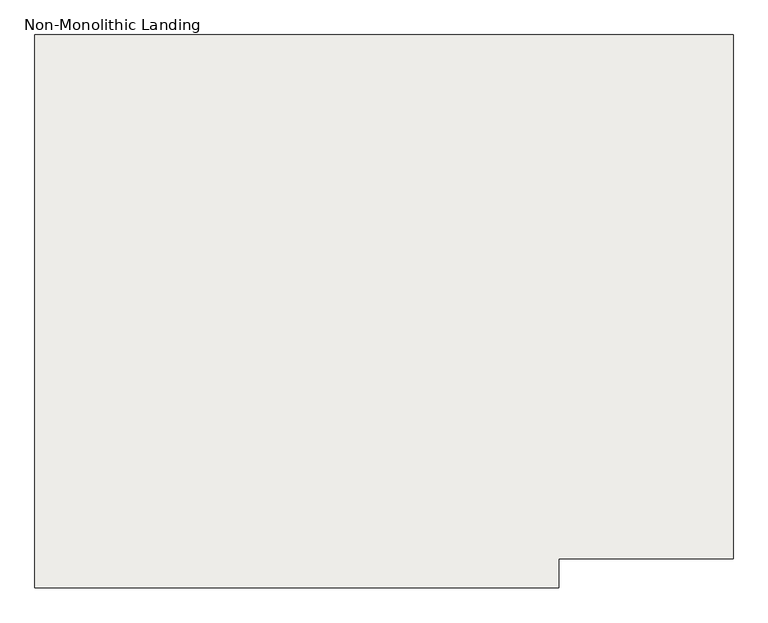
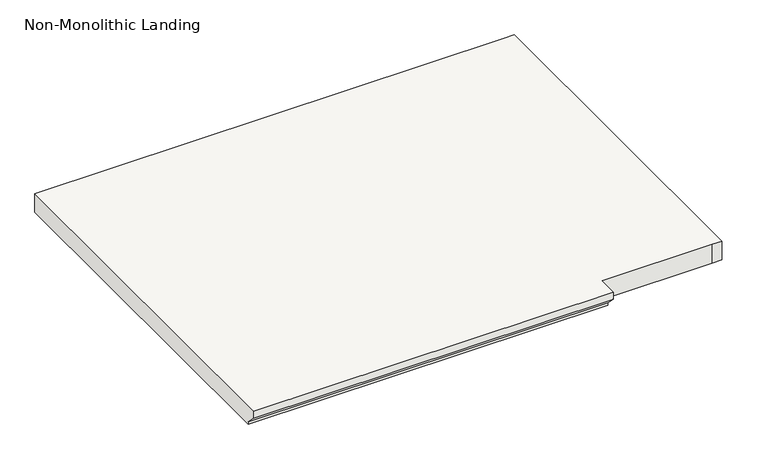
"""IFC4 building model written with IfcOpenShell, lengths in millimetres: slab geometry, Non-Monolithic Landing."""

from ifc_helpers import new_model, si_unit, origin, place, context, project, spatial, faceted_brep, source, transform, mapped, element, save


def non_monolithic_landing_ccb861af(model_context):
    return source(origin(), model_context, "Body", "Brep", [
        faceted_brep([(-12728.1167709, 2715.8362133, 1225.55), (-12728.1167709, 2715.8362133, 1244.6), (-13642.5167709, 2715.8362133, 1244.6), (-13642.5167709, 2715.8362133, 1225.55), (-12728.1167709, 2741.2362133, 1200.15), (-13642.5167709, 2741.2362133, 1200.15), (-12728.1167709, 2766.6362133, 1244.6), (-12448.7167709, 2766.6362133, 1244.6), (-12423.3167709, 2766.6362133, 1244.6), (-12423.3167709, 3681.0362133, 1244.6), (-12448.7167709, 3681.0362133, 1244.6), (-13642.5167709, 3681.0362133, 1244.6), (-12728.1167709, 2741.2362133, 1193.8), (-13642.5167709, 2741.2362133, 1193.8), (-13642.5167709, 3681.0362133, 1193.8), (-12448.7167709, 3681.0362133, 1193.8), (-12423.3167709, 3681.0362133, 1193.8), (-12423.3167709, 2766.6362133, 1193.8), (-12448.7167709, 2766.6362133, 1193.8), (-12728.1167709, 2766.6362133, 1193.8)], [[[0, 1, 2, 3]], [[4, 0, 3, 5]], [[6, 7, 8, 9, 10, 11, 2, 1]], [[12, 13, 14, 15, 16, 17, 18, 19]], [[13, 12, 4, 5]], [[6, 1, 0, 4, 12, 19]], [[7, 6, 19, 18]], [[8, 7, 18, 17]], [[9, 8, 17, 16]], [[10, 9, 16, 15]], [[11, 10, 15, 14]], [[2, 11, 14, 13, 5, 3]]]),
    ])


if __name__ == "__main__":
    model = new_model("IFC4")
    model_context = context("Model", 3, world=origin())
    ifc_project = project(units=[si_unit("LENGTHUNIT", "METRE", prefix="MILLI")], contexts=[model_context])
    site = spatial("IfcSite", under=ifc_project)
    building = spatial("IfcBuilding", under=site)
    placement = place(None, origin())
    non_monolithic_landing_shape = non_monolithic_landing_ccb861af(model_context)
    element("IfcSlab", 1, ObjectType="Non-Monolithic Landing", at=placement, inside=building, context=model_context, shape_type="MappedRepresentation", body=[
        mapped(non_monolithic_landing_shape, transform((0.0, 0.0, 0.0), x_axis=(1.0, 0.0, 0.0), y_axis=(0.0, 1.0, 0.0), z_axis=(0.0, 0.0, 1.0))),
    ])
    save(model, "model.ifc")
